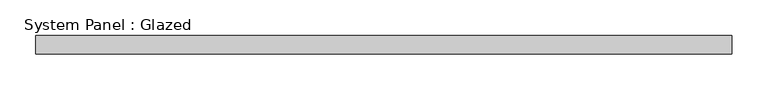
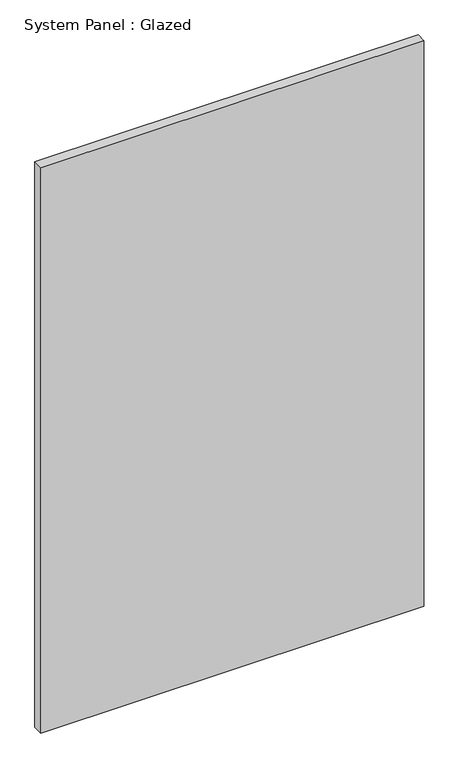
"""IFC4 building model written with IfcOpenShell, lengths in millimetres: plate geometry, System Panel : Glazed."""

from ifc_helpers import new_model, si_unit, origin, origin_with_axes, place, context, project, spatial, polyline, outline, extrude, source, transform, mapped, element, save


def system_panel_glazed_daa3f2c1(model_context):
    return source(origin(), model_context, "Body", "SweptSolid", [
        extrude(outline(polyline([(485.775, 19.05), (-485.775, 19.05), (-485.775, 44.45), (485.775, 44.45), (485.775, 19.05)])), origin_with_axes(), (0.0, 0.0, 1.0), 1515.7479304),
    ])


if __name__ == "__main__":
    model = new_model("IFC4")
    model_context = context("Model", 3, world=origin())
    ifc_project = project(units=[si_unit("LENGTHUNIT", "METRE", prefix="MILLI")], contexts=[model_context])
    site = spatial("IfcSite", under=ifc_project)
    building = spatial("IfcBuilding", under=site)
    placement = place(None, origin())
    system_panel_glazed_shape = system_panel_glazed_daa3f2c1(model_context)
    element("IfcPlate", 1, ObjectType="System Panel : Glazed", at=placement, inside=building, context=model_context, shape_type="MappedRepresentation", body=[
        mapped(system_panel_glazed_shape, transform((0.0, 0.0, 0.0), x_axis=(1.0, 0.0, 0.0), y_axis=(0.0, 1.0, 0.0), z_axis=(0.0, 0.0, 1.0))),
    ])
    save(model, "model.ifc")

# Revit data of these elements
# Type "System Panel : Glazed"
#   Construction Type Id = "GSP4R"
#   Analytic Construction = "1/8 in Pilkington single glazing"
#   Visual Light Transmittance = 0.9
#   Solar Heat Gain Coefficient = 0.86
#   Heat Transfer Coefficient (U) = 1.18115 BTU/(h·ft²·°F)
#   Define Thermal Properties by = 1
# Element 1 (IfcPlate, "System Panel : Glazed")
#   Materials on its faces: "Glass"
# Materials
#   "Glass": class "Glass", colour RGB 0 128 192, transparency 0.75, Description = "Soda Lime Glass", Cost = 0
